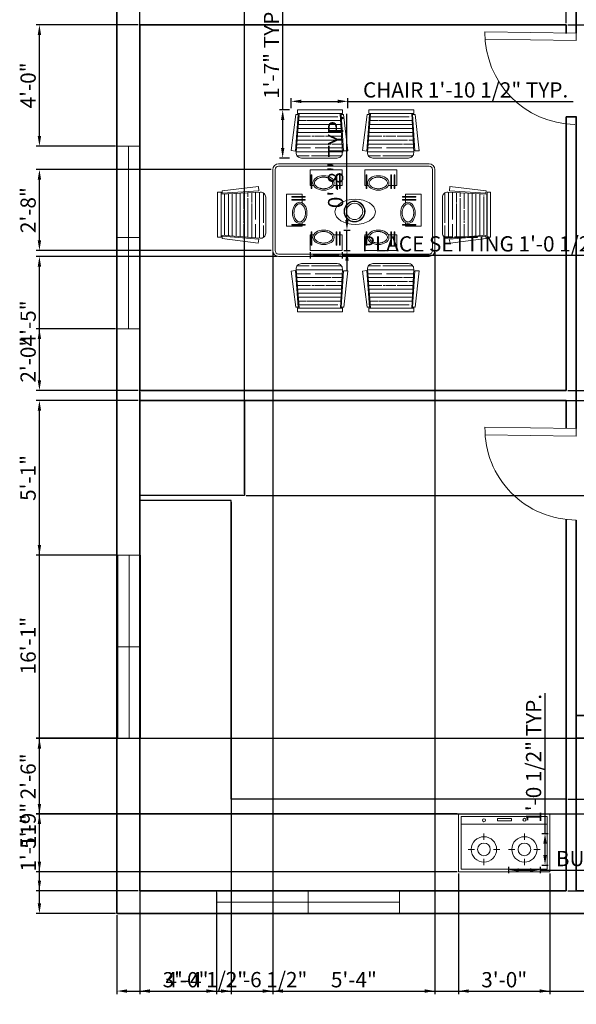
# Model space of a CAD drawing. Units: inches. Extents: x 1973 to 2661, y 1730 to 2412.
# Tile 1 of 5: x 1978 to 2197, y 1730 to 2117. Entities that reach past the tile are written whole.
import ezdxf

# ---------------------------------------------------------------- set-up
doc = ezdxf.new("R2010")
doc.units = ezdxf.units.IN
for name, color, linetype, lineweight in [('A-ANNO-DIMS', 2, 'Continuous', 18), ('A-DOOR', 3, 'Continuous', 18), ('A-EQPM', 9, 'Continuous', 18), ('A-FLOR-CASE', 32, 'Continuous', 25), ('A-FURN', 8, 'Continuous', 18), ('A-GLAZ', 4, 'Continuous', 18), ('A-WALL', 7, 'Continuous', 35)]:
    doc.layers.add(name, color=color, linetype=linetype, lineweight=lineweight)
doc.styles.get("Standard").update_dxf_attribs({"font": 'arial.ttf'})
doc.dimstyles.new('ISO-25', dxfattribs={"dimtxt": 6, "dimasz": 4, "dimexe": 1.25, "dimexo": 0.625, "dimtad": 1, "dimdec": 0, "dimrnd": 6, "dimlunit": 3, "dimtxsty": 'Standard', "dimcen": 2.5, "dimadec": 0, "dimazin": 0, "dimtfac": 1, "dimtdec": 0, "dimtmove": 0, "dimatfit": 3, "dimfxl": 1, "dimarcsym": 0})

# ---------------------------------------------------------------- blocks, each defined once
blk = doc.blocks.new('WIN-72-TWO-LIGHT')
for p, q in [((0, 72), (9, 72)), ((0, 0), (0, 72)), ((4.5, 72), (4.5, 36)), ((9, 72), (9, 0)), ((4.5, 36), (0, 36)), ((0, 36), (9, 36)), ((4.5, 36), (4.5, 0)), ((9, 0), (0, 0))]:
    blk.add_line(p, q)
blk = doc.blocks.new('CHAIR-DINING-SLATTED')
for p, q in [((0, 3.05), (1.85, 17.22)), ((2.79, 17.13), (1.68, 2.71)), ((1.85, 17.22), (2.79, 17.13)), ((1.98, 2.21), (3.17, 17.52)), ((2.47, 17.6), (2.47, 18.99)), ((2.47, 18.99), (20.19, 18.99)), ((20.19, 17.6), (2.47, 17.6)), ((3.07, 16.28), (18.38, 16.28)), ((18.88, 16.28), (18.96, 16.28)), ((19.37, 17.52), (20.16, 2.16)), ((20.68, 17.22), (19.74, 17.13)), ((19.74, 17.13), (20.61, 2.8)), ((20.19, 18.99), (20.19, 17.6)), ((22.33, 2.88), (20.68, 17.22)), ((2.72, 11.67), (19.67, 11.67)), ((2.83, 13.21), (19.59, 13.21)), ((2.95, 14.75), (6.04, 14.75)), ((6.28, 14.75), (19.51, 14.75)), ((2.48, 8.59), (7.56, 8.59)), ((2.6, 10.13), (19.75, 10.13)), ((8.13, 8.59), (8.91, 8.59)), ((9.16, 8.59), (13.09, 8.59)), ((13.59, 8.59), (19.83, 8.59)), ((2.12, 3.98), (7.56, 3.98)), ((2.24, 5.52), (15.72, 5.52)), ((2.36, 7.06), (17.73, 7.06)), ((9.4, 3.98), (20.07, 3.98)), ((16.09, 5.52), (19.99, 5.52)), ((18.26, 7.06), (19.91, 7.06)), ((1.68, 2.71), (0, 3.05)), ((2, 2.44), (20.15, 2.44)), ((2.33, 0.9), (7.06, 0.9)), ((18.11, 0), (4.03, 0)), ((8.05, 0.9), (19.81, 0.9)), ((20.61, 2.8), (22.33, 2.88))]:
    blk.add_line(p, q)
for centre, start, end in [((4.03, 2.05), 175.5808, 270), ((18.11, 2.05), 270, 2.9494)]:
    blk.add_arc(centre, 2.05, start, end)
blk = doc.blocks.new('DINING-PLACE-SETTING')
for p, q in [((0, 0), (0, 6.2)), ((0, 6.2), (1.33, 6.2)), ((0.44, 2.07), (0.44, 7.38)), ((0.44, 7.38), (0.7, 7.38)), ((0.7, 7.38), (0.7, 2.07)), ((9.19, 6.2), (12.59, 6.2)), ((10.26, 2.07), (10.26, 7.38)), ((10.26, 7.38), (10.52, 7.38)), ((10.52, 7.38), (10.52, 2.07)), ((11.48, 2.07), (11.48, 7.38)), ((11.48, 7.38), (11.74, 7.38)), ((11.74, 7.38), (11.74, 2.07)), ((12.59, 6.2), (12.59, 0)), ((12.59, 0), (0, 0)), ((0.7, 2.07), (0.44, 2.07)), ((10.52, 2.07), (10.26, 2.07)), ((11.74, 2.07), (11.48, 2.07))]:
    blk.add_line(p, q)
blk.add_ellipse((5.26, 5.21), major_axis=(4.19, 0), ratio=0.682819)
blk.add_open_spline([(8.86, 5.21), (8.86, 5.36), (8.83, 5.53), (8.71, 5.87), (8.6, 6.05), (8.39, 6.32), (8.3, 6.41), (8.11, 6.58), (8.01, 6.66), (7.66, 6.9), (7.39, 7.04), (6.95, 7.21), (6.8, 7.25), (6.5, 7.34), (6.34, 7.37), (6.03, 7.42), (5.87, 7.44), (5.56, 7.47), (5.42, 7.48), (5.1, 7.48), (4.96, 7.47), (4.65, 7.44), (4.49, 7.42), (4.18, 7.37), (4.03, 7.34), (3.72, 7.25), (3.57, 7.21), (3.13, 7.04), (2.86, 6.9), (2.52, 6.66), (2.41, 6.58), (2.22, 6.41), (2.14, 6.32), (1.92, 6.05), (1.82, 5.87), (1.69, 5.53), (1.66, 5.36), (1.66, 5.05), (1.69, 4.88), (1.82, 4.54), (1.92, 4.36), (2.14, 4.09), (2.22, 4), (2.41, 3.83), (2.52, 3.75), (2.86, 3.51), (3.13, 3.37), (3.57, 3.21), (3.72, 3.16), (4.03, 3.07), (4.18, 3.04), (4.49, 2.99), (4.65, 2.97), (4.96, 2.94), (5.1, 2.94), (5.42, 2.94), (5.56, 2.94), (5.87, 2.97), (6.03, 2.99), (6.34, 3.04), (6.5, 3.07), (6.8, 3.16), (6.95, 3.21), (7.39, 3.37), (7.66, 3.51), (8.01, 3.75), (8.11, 3.83), (8.3, 4), (8.39, 4.09), (8.6, 4.36), (8.71, 4.54), (8.83, 4.88), (8.86, 5.05), (8.86, 5.21)], degree=3, knots=[0, 0, 0, 0, 0.261799, 0.261799, 0.523599, 0.523599, 0.654498, 0.654498, 0.785398, 0.785398, 1.047198, 1.047198, 1.178097, 1.178097, 1.308997, 1.308997, 1.439897, 1.439897, 1.570796, 1.570796, 1.701696, 1.701696, 1.832596, 1.832596, 1.963495, 1.963495, 2.094395, 2.094395, 2.356194, 2.356194, 2.487094, 2.487094, 2.617994, 2.617994, 2.879793, 2.879793, 3.141593, 3.141593, 3.403392, 3.403392, 3.665191, 3.665191, 3.796091, 3.796091, 3.926991, 3.926991, 4.18879, 4.18879, 4.31969, 4.31969, 4.45059, 4.45059, 4.581489, 4.581489, 4.712389, 4.712389, 4.843289, 4.843289, 4.974188, 4.974188, 5.105088, 5.105088, 5.235988, 5.235988, 5.497787, 5.497787, 5.628687, 5.628687, 5.759587, 5.759587, 6.021386, 6.021386, 6.283185, 6.283185, 6.283185, 6.283185])
blk = doc.blocks.new('COOKTOP-BURNER')
for p, q in [((6.24, 9.98), (6.24, 12.48)), ((2.5, 6.24), (0, 6.24)), ((12.48, 6.24), (9.98, 6.24)), ((6.24, 0), (6.24, 2.5))]:
    blk.add_line(p, q)
for radius in [4.99, 2.5]:
    blk.add_circle((6.24, 6.24), radius)
blk = doc.blocks.new('*D16')
at = {"layer": 'A-ANNO-DIMS', "color": 0, "lineweight": -2, "transparency": 16777216}
for p, q in [((2092.18, 2025.82), (2092.18, 2023.31)), ((2096.18, 2024.56), (2100.77, 2024.56)), ((2104.77, 2025.82), (2104.77, 2023.31)), ((2104.77, 2024.56), (2228.74, 2024.56))]:
    blk.add_line(p, q, dxfattribs=at)
at = {"layer": 'A-ANNO-DIMS', "color": 0, "transparency": 16777216}
for points in [[(2096.18, 2025.23), (2096.18, 2023.89), (2092.18, 2024.56)], [(2100.77, 2025.23), (2100.77, 2023.89), (2104.77, 2024.56)]]:
    blk.add_solid(points, dxfattribs=at)
at = {"layer": 'Defpoints', "color": 0, "transparency": 16777216}
for p in [(2092.18, 2026.45), (2104.77, 2026.45), (2104.77, 2024.56)]:
    blk.add_point(p, dxfattribs=at)
at = {"layer": 'A-ANNO-DIMS', "color": 0, "transparency": 16777216, "insert": (2168.76, 2028.29), "char_height": 6, "attachment_point": 5}
blk.add_mtext('PLACE SETTING 1\'-0 1/2" TYP.', dxfattribs=at)
blk = doc.blocks.new('*D17')
at = {"layer": 'A-ANNO-DIMS', "color": 0, "lineweight": -2, "transparency": 16777216}
for p, q in [((2106.66, 2038.51), (2106.66, 2080.34)), ((2105.4, 2034.51), (2107.91, 2034.51)), ((2106.66, 2026.45), (2106.66, 2034.51)), ((2105.4, 2026.45), (2107.91, 2026.45)), ((2106.66, 2022.45), (2106.66, 2018.45))]:
    blk.add_line(p, q, dxfattribs=at)
at = {"layer": 'A-ANNO-DIMS', "color": 0, "transparency": 16777216}
for points in [[(2105.99, 2038.51), (2107.33, 2038.51), (2106.66, 2034.51)], [(2105.99, 2022.45), (2107.33, 2022.45), (2106.66, 2026.45)]]:
    blk.add_solid(points, dxfattribs=at)
at = {"layer": 'Defpoints', "color": 0, "transparency": 16777216}
for p in [(2104.77, 2034.51), (2106.66, 2034.51), (2104.77, 2026.45)]:
    blk.add_point(p, dxfattribs=at)
at = {"layer": 'A-ANNO-DIMS', "color": 0, "transparency": 16777216, "insert": (2102.97, 2061.43), "char_height": 6, "attachment_point": 5, "rotation": 90}
blk.add_mtext('0\'-8" TYP.', dxfattribs=at)
blk = doc.blocks.new('*D20')
at = {"layer": 'A-ANNO-DIMS', "color": 0, "lineweight": -2, "transparency": 16777216}
for p, q in [((2084.68, 2082.47), (2084.68, 2086.44)), ((2107.02, 2082.47), (2107.02, 2086.44)), ((2088.68, 2085.19), (2103.02, 2085.19)), ((2107.02, 2085.19), (2195.82, 2085.19))]:
    blk.add_line(p, q, dxfattribs=at)
at = {"layer": 'A-ANNO-DIMS', "color": 0, "transparency": 16777216}
for points in [[(2088.68, 2085.86), (2088.68, 2084.53), (2084.68, 2085.19)], [(2103.02, 2085.86), (2103.02, 2084.53), (2107.02, 2085.19)]]:
    blk.add_solid(points, dxfattribs=at)
at = {"layer": 'Defpoints', "color": 0, "transparency": 16777216}
for p in [(2107.02, 2085.19), (2084.68, 2081.84), (2107.02, 2081.84)]:
    blk.add_point(p, dxfattribs=at)
at = {"layer": 'A-ANNO-DIMS', "color": 0, "transparency": 16777216, "insert": (2153.42, 2088.92), "char_height": 6, "attachment_point": 5}
blk.add_mtext('CHAIR 1\'-10 1/2" TYP.', dxfattribs=at)
blk = doc.blocks.new('*D21')
at = {"layer": 'A-ANNO-DIMS', "color": 0, "lineweight": -2, "transparency": 16777216}
for p, q in [((2081.33, 2081.84), (2081.33, 2123.1)), ((2084.06, 2081.84), (2080.08, 2081.84)), ((2081.33, 2066.85), (2081.33, 2077.84)), ((2084.06, 2062.85), (2080.08, 2062.85))]:
    blk.add_line(p, q, dxfattribs=at)
at = {"layer": 'A-ANNO-DIMS', "color": 0, "transparency": 16777216}
for points in [[(2080.67, 2077.84), (2082, 2077.84), (2081.33, 2081.84)], [(2080.67, 2066.85), (2082, 2066.85), (2081.33, 2062.85)]]:
    blk.add_solid(points, dxfattribs=at)
at = {"layer": 'Defpoints', "color": 0, "transparency": 16777216}
for p in [(2081.33, 2081.84), (2084.68, 2081.84), (2084.68, 2062.85)]:
    blk.add_point(p, dxfattribs=at)
at = {"layer": 'A-ANNO-DIMS', "color": 0, "transparency": 16777216, "insert": (2077.7, 2104.47), "char_height": 6, "attachment_point": 5, "rotation": 90}
blk.add_mtext('1\'-7" TYP.', dxfattribs=at)
blk = doc.blocks.new('*D28')
at = {"layer": 'A-ANNO-DIMS', "color": 0, "lineweight": -2, "transparency": 16777216}
for p, q in [((2170.36, 1783.74), (2170.36, 1781.24)), ((2182.84, 1783.74), (2182.84, 1781.24)), ((2174.36, 1782.49), (2178.84, 1782.49)), ((2182.84, 1782.49), (2276.1, 1782.49))]:
    blk.add_line(p, q, dxfattribs=at)
at = {"layer": 'A-ANNO-DIMS', "color": 0, "transparency": 16777216}
for points in [[(2174.36, 1783.16), (2174.36, 1781.83), (2170.36, 1782.49)], [(2178.84, 1783.16), (2178.84, 1781.83), (2182.84, 1782.49)]]:
    blk.add_solid(points, dxfattribs=at)
at = {"layer": 'Defpoints', "color": 0, "transparency": 16777216}
for p in [(2170.36, 1784.36), (2182.84, 1784.36), (2182.84, 1782.49)]:
    blk.add_point(p, dxfattribs=at)
at = {"layer": 'A-ANNO-DIMS', "color": 0, "transparency": 16777216, "insert": (2231.47, 1786.22), "char_height": 6, "attachment_point": 5}
blk.add_mtext('BURNER 1\'-0 1/2" TYP.', dxfattribs=at)
blk = doc.blocks.new('*D29')
at = {"layer": 'A-ANNO-DIMS', "color": 0, "lineweight": -2, "transparency": 16777216}
for p, q in [((2184.71, 1796.84), (2184.71, 1852.08)), ((2183.47, 1796.84), (2185.96, 1796.84)), ((2184.71, 1788.36), (2184.71, 1792.84)), ((2183.47, 1784.36), (2185.96, 1784.36))]:
    blk.add_line(p, q, dxfattribs=at)
at = {"layer": 'A-ANNO-DIMS', "color": 0, "transparency": 16777216}
for points in [[(2184.05, 1792.84), (2185.38, 1792.84), (2184.71, 1796.84)], [(2184.05, 1788.36), (2185.38, 1788.36), (2184.71, 1784.36)]]:
    blk.add_solid(points, dxfattribs=at)
at = {"layer": 'Defpoints', "color": 0, "transparency": 16777216}
for p in [(2182.84, 1796.84), (2184.71, 1796.84), (2182.84, 1784.36)]:
    blk.add_point(p, dxfattribs=at)
at = {"layer": 'A-ANNO-DIMS', "color": 0, "transparency": 16777216, "insert": (2180.98, 1826.46), "char_height": 6, "attachment_point": 5, "rotation": 90}
blk.add_mtext('1\'-0 1/2" TYP.', dxfattribs=at)
blk = doc.blocks.new('*D30')
at = {"layer": 'A-ANNO-DIMS', "color": 0, "lineweight": -2, "transparency": 16777216}
for p, q in [((2016.04, 1764.73), (2016.04, 1733.57)), ((2616.04, 1764.73), (2616.04, 1733.57)), ((2020.04, 1734.82), (2612.04, 1734.82))]:
    blk.add_line(p, q, dxfattribs=at)
at = {"layer": 'A-ANNO-DIMS', "color": 0, "transparency": 16777216}
for points in [[(2020.04, 1735.49), (2020.04, 1734.15), (2016.04, 1734.82)], [(2612.04, 1735.49), (2612.04, 1734.15), (2616.04, 1734.82)]]:
    blk.add_solid(points, dxfattribs=at)
at = {"layer": 'Defpoints', "color": 0, "transparency": 16777216}
for p in [(2016.04, 1765.35), (2616.04, 1765.35), (2616.04, 1734.82)]:
    blk.add_point(p, dxfattribs=at)
at = {"layer": 'A-ANNO-DIMS', "color": 0, "transparency": 16777216, "insert": (2316.04, 1738.51), "char_height": 6, "attachment_point": 5}
blk.add_mtext('50\'-0"', dxfattribs=at)
blk = doc.blocks.new('*D40')
at = {"layer": 'A-ANNO-DIMS', "color": 0, "lineweight": -2, "transparency": 16777216}
for p, q in [((2015.71, 1834.42), (1984.22, 1834.42)), ((1985.47, 1769.35), (1985.47, 1830.42)), ((2015.42, 1765.35), (1984.22, 1765.35))]:
    blk.add_line(p, q, dxfattribs=at)
at = {"layer": 'A-ANNO-DIMS', "color": 0, "transparency": 16777216}
for points in [[(1984.81, 1830.42), (1986.14, 1830.42), (1985.47, 1834.42)], [(1984.81, 1769.35), (1986.14, 1769.35), (1985.47, 1765.35)]]:
    blk.add_solid(points, dxfattribs=at)
at = {"layer": 'Defpoints', "color": 0, "transparency": 16777216}
for p in [(1985.47, 1834.42), (2016.33, 1834.42), (2016.04, 1765.35)]:
    blk.add_point(p, dxfattribs=at)
at = {"layer": 'A-ANNO-DIMS', "color": 0, "transparency": 16777216, "insert": (1981.79, 1799.89), "char_height": 6, "attachment_point": 5, "rotation": 90}
blk.add_mtext('5\'-9"', dxfattribs=at)
blk = doc.blocks.new('*D41')
at = {"layer": 'A-ANNO-DIMS', "color": 0, "lineweight": -2, "transparency": 16777216}
for p, q in [((2024.42, 1967.35), (1984.22, 1967.35)), ((1985.47, 1910.42), (1985.47, 1963.35)), ((2015.71, 1906.42), (1984.22, 1906.42))]:
    blk.add_line(p, q, dxfattribs=at)
at = {"layer": 'A-ANNO-DIMS', "color": 0, "transparency": 16777216}
for points in [[(1984.81, 1963.35), (1986.14, 1963.35), (1985.47, 1967.35)], [(1984.81, 1910.42), (1986.14, 1910.42), (1985.47, 1906.42)]]:
    blk.add_solid(points, dxfattribs=at)
at = {"layer": 'Defpoints', "color": 0, "transparency": 16777216}
for p in [(1985.47, 1967.35), (2025.04, 1967.35), (2016.33, 1906.42)]:
    blk.add_point(p, dxfattribs=at)
at = {"layer": 'A-ANNO-DIMS', "color": 0, "transparency": 16777216, "insert": (1981.79, 1936.89), "char_height": 6, "attachment_point": 5, "rotation": 90}
blk.add_mtext('5\'-1"', dxfattribs=at)
blk = doc.blocks.new('*D42')
at = {"layer": 'A-ANNO-DIMS', "color": 0, "lineweight": -2, "transparency": 16777216}
for p, q in [((2015.49, 1995.59), (1984.22, 1995.59)), ((1985.47, 1975.35), (1985.47, 1991.59)), ((2024.42, 1971.35), (1984.22, 1971.35))]:
    blk.add_line(p, q, dxfattribs=at)
at = {"layer": 'A-ANNO-DIMS', "color": 0, "transparency": 16777216}
for points in [[(1984.81, 1991.59), (1986.14, 1991.59), (1985.47, 1995.59)], [(1984.81, 1975.35), (1986.14, 1975.35), (1985.47, 1971.35)]]:
    blk.add_solid(points, dxfattribs=at)
at = {"layer": 'Defpoints', "color": 0, "transparency": 16777216}
for p in [(1985.47, 1995.59), (2016.11, 1995.59), (2025.04, 1971.35)]:
    blk.add_point(p, dxfattribs=at)
at = {"layer": 'A-ANNO-DIMS', "color": 0, "transparency": 16777216, "insert": (1981.79, 1983.47), "char_height": 6, "attachment_point": 5, "rotation": 90}
blk.add_mtext('2\'-0"', dxfattribs=at)
blk = doc.blocks.new('*D43')
at = {"layer": 'A-ANNO-DIMS', "color": 0, "lineweight": -2, "transparency": 16777216}
for p, q in [((2024.42, 2115.35), (1984.22, 2115.35)), ((1985.47, 2071.59), (1985.47, 2111.35)), ((2015.49, 2067.59), (1984.22, 2067.59))]:
    blk.add_line(p, q, dxfattribs=at)
at = {"layer": 'A-ANNO-DIMS', "color": 0, "transparency": 16777216}
for points in [[(1984.81, 2111.35), (1986.14, 2111.35), (1985.47, 2115.35)], [(1984.81, 2071.59), (1986.14, 2071.59), (1985.47, 2067.59)]]:
    blk.add_solid(points, dxfattribs=at)
at = {"layer": 'Defpoints', "color": 0, "transparency": 16777216}
for p in [(1985.47, 2115.35), (2025.04, 2115.35), (2016.11, 2067.59)]:
    blk.add_point(p, dxfattribs=at)
at = {"layer": 'A-ANNO-DIMS', "color": 0, "transparency": 16777216, "insert": (1981.79, 2091.47), "char_height": 6, "attachment_point": 5, "rotation": 90}
blk.add_mtext('4\'-0"', dxfattribs=at)
blk = doc.blocks.new('*D46')
at = {"layer": 'A-ANNO-DIMS', "color": 0, "lineweight": -2, "transparency": 16777216}
for p, q in [((2025.04, 2115.98), (2025.04, 2397.1)), ((2193.04, 2115.98), (2193.04, 2397.1)), ((2029.04, 2395.85), (2189.04, 2395.85))]:
    blk.add_line(p, q, dxfattribs=at)
at = {"layer": 'A-ANNO-DIMS', "color": 0, "transparency": 16777216}
for points in [[(2029.04, 2396.52), (2029.04, 2395.18), (2025.04, 2395.85)], [(2189.04, 2396.52), (2189.04, 2395.18), (2193.04, 2395.85)]]:
    blk.add_solid(points, dxfattribs=at)
at = {"layer": 'Defpoints', "color": 0, "transparency": 16777216}
for p in [(2193.04, 2395.85), (2025.04, 2115.35), (2193.04, 2115.35)]:
    blk.add_point(p, dxfattribs=at)
at = {"layer": 'A-ANNO-DIMS', "color": 0, "transparency": 16777216, "insert": (2109.04, 2399.54), "char_height": 6, "attachment_point": 5}
blk.add_mtext('14\'-0"', dxfattribs=at)
blk = doc.blocks.new('*D55')
at = {"layer": 'A-ANNO-DIMS', "color": 0, "lineweight": -2, "transparency": 16777216}
for p, q in [((2025.04, 1927.35), (2025.04, 1733.57)), ((2061.04, 1927.35), (2061.04, 1733.57)), ((2029.04, 1734.82), (2057.04, 1734.82))]:
    blk.add_line(p, q, dxfattribs=at)
at = {"layer": 'A-ANNO-DIMS', "color": 0, "transparency": 16777216}
for points in [[(2029.04, 1735.49), (2029.04, 1734.15), (2025.04, 1734.82)], [(2057.04, 1735.49), (2057.04, 1734.15), (2061.04, 1734.82)]]:
    blk.add_solid(points, dxfattribs=at)
at = {"layer": 'Defpoints', "color": 0, "transparency": 16777216}
for p in [(2025.04, 1927.97), (2061.04, 1927.97), (2061.04, 1734.82)]:
    blk.add_point(p, dxfattribs=at)
at = {"layer": 'A-ANNO-DIMS', "color": 0, "transparency": 16777216, "insert": (2043.04, 1738.51), "char_height": 6, "attachment_point": 5}
blk.add_mtext('3\'-0"', dxfattribs=at)
blk = doc.blocks.new('*D56')
at = {"layer": 'A-ANNO-DIMS', "color": 0, "lineweight": -2, "transparency": 16777216}
for p, q in [((2025.04, 1773.73), (2025.04, 1733.57)), ((2055.31, 1773.69), (2055.31, 1733.57)), ((2029.04, 1734.82), (2051.31, 1734.82)), ((2055.31, 1734.82), (2090.6, 1734.82))]:
    blk.add_line(p, q, dxfattribs=at)
at = {"layer": 'A-ANNO-DIMS', "color": 0, "transparency": 16777216}
for points in [[(2029.04, 1735.49), (2029.04, 1734.15), (2025.04, 1734.82)], [(2051.31, 1735.49), (2051.31, 1734.15), (2055.31, 1734.82)]]:
    blk.add_solid(points, dxfattribs=at)
at = {"layer": 'Defpoints', "color": 0, "transparency": 16777216}
for p in [(2025.04, 1774.35), (2055.31, 1774.32), (2055.31, 1734.82)]:
    blk.add_point(p, dxfattribs=at)
at = {"layer": 'A-ANNO-DIMS', "color": 0, "transparency": 16777216, "insert": (2074.95, 1738.55), "char_height": 6, "attachment_point": 5}
blk.add_mtext('2\'-6 1/2"', dxfattribs=at)
blk = doc.blocks.new('*D57')
at = {"layer": 'A-ANNO-DIMS', "color": 0, "lineweight": -2, "transparency": 16777216}
for p, q in [((2193.67, 1810.35), (2647.79, 1810.35)), ((2646.54, 1778.35), (2646.54, 1806.35)), ((2193.67, 1774.35), (2647.79, 1774.35))]:
    blk.add_line(p, q, dxfattribs=at)
at = {"layer": 'A-ANNO-DIMS', "color": 0, "transparency": 16777216}
for points in [[(2645.88, 1806.35), (2647.21, 1806.35), (2646.54, 1810.35)], [(2645.88, 1778.35), (2647.21, 1778.35), (2646.54, 1774.35)]]:
    blk.add_solid(points, dxfattribs=at)
at = {"layer": 'Defpoints', "color": 0, "transparency": 16777216}
for p in [(2193.04, 1810.35), (2646.54, 1810.35), (2193.04, 1774.35)]:
    blk.add_point(p, dxfattribs=at)
at = {"layer": 'A-ANNO-DIMS', "color": 0, "transparency": 16777216, "insert": (2642.85, 1792.35), "char_height": 6, "attachment_point": 5, "rotation": 90}
blk.add_mtext('3\'-0"', dxfattribs=at)
blk = doc.blocks.new('*D58')
at = {"layer": 'A-ANNO-DIMS', "color": 0, "lineweight": -2, "transparency": 16777216}
for p, q in [((2024.42, 1967.35), (1984.22, 1967.35)), ((1985.47, 1778.35), (1985.47, 1963.35)), ((2024.42, 1774.35), (1984.22, 1774.35))]:
    blk.add_line(p, q, dxfattribs=at)
at = {"layer": 'A-ANNO-DIMS', "color": 0, "transparency": 16777216}
for points in [[(1984.81, 1963.35), (1986.14, 1963.35), (1985.47, 1967.35)], [(1984.81, 1778.35), (1986.14, 1778.35), (1985.47, 1774.35)]]:
    blk.add_solid(points, dxfattribs=at)
at = {"layer": 'Defpoints', "color": 0, "transparency": 16777216}
for p in [(1985.47, 1967.35), (2025.04, 1967.35), (2025.04, 1774.35)]:
    blk.add_point(p, dxfattribs=at)
at = {"layer": 'A-ANNO-DIMS', "color": 0, "transparency": 16777216, "insert": (1981.79, 1870.85), "char_height": 6, "attachment_point": 5, "rotation": 90}
blk.add_mtext('16\'-1"', dxfattribs=at)
blk = doc.blocks.new('*D59')
at = {"layer": 'A-ANNO-DIMS', "color": 0, "lineweight": -2, "transparency": 16777216}
for p, q in [((2193.67, 2115.35), (2647.79, 2115.35)), ((2646.54, 1975.35), (2646.54, 2111.35)), ((2193.67, 1971.35), (2647.79, 1971.35))]:
    blk.add_line(p, q, dxfattribs=at)
at = {"layer": 'A-ANNO-DIMS', "color": 0, "transparency": 16777216}
for points in [[(2645.88, 2111.35), (2647.21, 2111.35), (2646.54, 2115.35)], [(2645.88, 1975.35), (2647.21, 1975.35), (2646.54, 1971.35)]]:
    blk.add_solid(points, dxfattribs=at)
at = {"layer": 'Defpoints', "color": 0, "transparency": 16777216}
for p in [(2193.04, 2115.35), (2646.54, 2115.35), (2193.04, 1971.35)]:
    blk.add_point(p, dxfattribs=at)
at = {"layer": 'A-ANNO-DIMS', "color": 0, "transparency": 16777216, "insert": (2642.85, 2043.35), "char_height": 6, "attachment_point": 5, "rotation": 90}
blk.add_mtext('12\'-0"', dxfattribs=at)
blk = doc.blocks.new('*D64')
at = {"layer": 'A-ANNO-DIMS', "color": 0, "lineweight": -2, "transparency": 16777216}
for p, q in [((2324.17, 1834.25), (1984.22, 1834.25)), ((1985.47, 1808.45), (1985.47, 1830.25)), ((2324.17, 1804.45), (1984.22, 1804.45))]:
    blk.add_line(p, q, dxfattribs=at)
at = {"layer": 'A-ANNO-DIMS', "color": 0, "transparency": 16777216}
for points in [[(1984.81, 1830.25), (1986.14, 1830.25), (1985.47, 1834.25)], [(1984.81, 1808.45), (1986.14, 1808.45), (1985.47, 1804.45)]]:
    blk.add_solid(points, dxfattribs=at)
at = {"layer": 'Defpoints', "color": 0, "transparency": 16777216}
for p in [(1985.47, 1834.25), (2324.79, 1834.25), (2324.79, 1804.45)]:
    blk.add_point(p, dxfattribs=at)
at = {"layer": 'A-ANNO-DIMS', "color": 0, "transparency": 16777216, "insert": (1981.79, 1819.35), "char_height": 6, "attachment_point": 5, "rotation": 90}
blk.add_mtext('2\'-6"', dxfattribs=at)
blk = doc.blocks.new('*D70')
at = {"layer": 'A-ANNO-DIMS', "color": 0, "lineweight": -2, "transparency": 16777216}
for p, q in [((2077.47, 2025.78), (2077.47, 1733.57)), ((2141.28, 2025.78), (2141.28, 1733.57)), ((2081.47, 1734.82), (2137.28, 1734.82))]:
    blk.add_line(p, q, dxfattribs=at)
at = {"layer": 'A-ANNO-DIMS', "color": 0, "transparency": 16777216}
for points in [[(2081.47, 1735.49), (2081.47, 1734.15), (2077.47, 1734.82)], [(2137.28, 1735.49), (2137.28, 1734.15), (2141.28, 1734.82)]]:
    blk.add_solid(points, dxfattribs=at)
at = {"layer": 'Defpoints', "color": 0, "transparency": 16777216}
for p in [(2077.47, 2026.4), (2141.28, 2026.4), (2141.28, 1734.82)]:
    blk.add_point(p, dxfattribs=at)
at = {"layer": 'A-ANNO-DIMS', "color": 0, "transparency": 16777216, "insert": (2109.38, 1738.5), "char_height": 6, "attachment_point": 5}
blk.add_mtext('5\'-4"', dxfattribs=at)
blk = doc.blocks.new('*D71')
at = {"layer": 'A-ANNO-DIMS', "color": 0, "lineweight": -2, "transparency": 16777216}
for p, q in [((2076.85, 2058.31), (1984.22, 2058.31)), ((1985.47, 2030.4), (1985.47, 2054.31)), ((2076.85, 2026.4), (1984.22, 2026.4))]:
    blk.add_line(p, q, dxfattribs=at)
at = {"layer": 'A-ANNO-DIMS', "color": 0, "transparency": 16777216}
for points in [[(1984.81, 2054.31), (1986.14, 2054.31), (1985.47, 2058.31)], [(1984.81, 2030.4), (1986.14, 2030.4), (1985.47, 2026.4)]]:
    blk.add_solid(points, dxfattribs=at)
at = {"layer": 'Defpoints', "color": 0, "transparency": 16777216}
for p in [(1985.47, 2058.31), (2077.47, 2058.31), (2077.47, 2026.4)]:
    blk.add_point(p, dxfattribs=at)
at = {"layer": 'A-ANNO-DIMS', "color": 0, "transparency": 16777216, "insert": (1981.79, 2042.35), "char_height": 6, "attachment_point": 5, "rotation": 90}
blk.add_mtext('2\'-8"', dxfattribs=at)
blk = doc.blocks.new('*D72')
at = {"layer": 'A-ANNO-DIMS', "color": 0, "lineweight": -2, "transparency": 16777216}
for p, q in [((2025.04, 1930.6), (2025.04, 2397.1)), ((2066.26, 1930.6), (2066.26, 2397.1)), ((2062.26, 2395.85), (2029.04, 2395.85))]:
    blk.add_line(p, q, dxfattribs=at)
at = {"layer": 'A-ANNO-DIMS', "color": 0, "transparency": 16777216}
for points in [[(2029.04, 2396.52), (2029.04, 2395.18), (2025.04, 2395.85)], [(2062.26, 2396.52), (2062.26, 2395.18), (2066.26, 2395.85)]]:
    blk.add_solid(points, dxfattribs=at)
at = {"layer": 'Defpoints', "color": 0, "transparency": 16777216}
for p in [(2025.04, 2395.85), (2025.04, 1929.97), (2066.26, 1929.97)]:
    blk.add_point(p, dxfattribs=at)
at = {"layer": 'A-ANNO-DIMS', "color": 0, "transparency": 16777216, "insert": (2045.65, 2399.54), "char_height": 6, "attachment_point": 5}
blk.add_mtext('3\'-5"', dxfattribs=at)
blk = doc.blocks.new('*D73')
at = {"layer": 'A-ANNO-DIMS', "color": 0, "lineweight": -2, "transparency": 16777216}
for p, q in [((2066.89, 1967.35), (2647.79, 1967.35)), ((2646.54, 1933.97), (2646.54, 1963.35)), ((2066.89, 1929.97), (2647.79, 1929.97))]:
    blk.add_line(p, q, dxfattribs=at)
at = {"layer": 'A-ANNO-DIMS', "color": 0, "transparency": 16777216}
for points in [[(2645.88, 1963.35), (2647.21, 1963.35), (2646.54, 1967.35)], [(2645.88, 1933.97), (2647.21, 1933.97), (2646.54, 1929.97)]]:
    blk.add_solid(points, dxfattribs=at)
at = {"layer": 'Defpoints', "color": 0, "transparency": 16777216}
for p in [(2066.26, 1967.35), (2646.54, 1967.35), (2066.26, 1929.97)]:
    blk.add_point(p, dxfattribs=at)
at = {"layer": 'A-ANNO-DIMS', "color": 0, "transparency": 16777216, "insert": (2642.81, 1948.66), "char_height": 6, "attachment_point": 5, "rotation": 90}
blk.add_mtext('3\'-1 1/2"', dxfattribs=at)
blk = doc.blocks.new('*D74')
at = {"layer": 'A-ANNO-DIMS', "color": 0, "lineweight": -2, "transparency": 16777216}
for p, q in [((2150.66, 1781.14), (2150.66, 1733.57)), ((2186.58, 1781.14), (2186.58, 1733.57)), ((2154.66, 1734.82), (2182.58, 1734.82))]:
    blk.add_line(p, q, dxfattribs=at)
at = {"layer": 'A-ANNO-DIMS', "color": 0, "transparency": 16777216}
for points in [[(2154.66, 1735.49), (2154.66, 1734.15), (2150.66, 1734.82)], [(2182.58, 1735.49), (2182.58, 1734.15), (2186.58, 1734.82)]]:
    blk.add_solid(points, dxfattribs=at)
at = {"layer": 'Defpoints', "color": 0, "transparency": 16777216}
for p in [(2150.66, 1781.77), (2186.58, 1781.77), (2186.58, 1734.82)]:
    blk.add_point(p, dxfattribs=at)
at = {"layer": 'A-ANNO-DIMS', "color": 0, "transparency": 16777216, "insert": (2168.62, 1738.51), "char_height": 6, "attachment_point": 5}
blk.add_mtext('3\'-0"', dxfattribs=at)
blk = doc.blocks.new('*D75')
at = {"layer": 'A-ANNO-DIMS', "color": 0, "lineweight": -2, "transparency": 16777216}
for p, q in [((2150.04, 1804.58), (1984.22, 1804.58)), ((1985.47, 1785.77), (1985.47, 1800.58)), ((2150.04, 1781.77), (1984.22, 1781.77))]:
    blk.add_line(p, q, dxfattribs=at)
at = {"layer": 'A-ANNO-DIMS', "color": 0, "transparency": 16777216}
for points in [[(1984.81, 1800.58), (1986.14, 1800.58), (1985.47, 1804.58)], [(1984.81, 1785.77), (1986.14, 1785.77), (1985.47, 1781.77)]]:
    blk.add_solid(points, dxfattribs=at)
at = {"layer": 'Defpoints', "color": 0, "transparency": 16777216}
for p in [(1985.47, 1804.58), (2150.66, 1804.58), (2150.66, 1781.77)]:
    blk.add_point(p, dxfattribs=at)
at = {"layer": 'A-ANNO-DIMS', "color": 0, "transparency": 16777216, "insert": (1981.84, 1793.17), "char_height": 6, "attachment_point": 5, "rotation": 90}
blk.add_mtext('1\'-11"', dxfattribs=at)
blk = doc.blocks.new('*D78')
at = {"layer": 'A-ANNO-DIMS', "color": 0, "lineweight": -2, "transparency": 16777216}
for p, q in [((2077.47, 2025.78), (2077.47, 1733.57)), ((2025.04, 1970.73), (2025.04, 1733.57)), ((2029.04, 1734.82), (2073.47, 1734.82))]:
    blk.add_line(p, q, dxfattribs=at)
at = {"layer": 'A-ANNO-DIMS', "color": 0, "transparency": 16777216}
for points in [[(2029.04, 1735.49), (2029.04, 1734.15), (2025.04, 1734.82)], [(2073.47, 1735.49), (2073.47, 1734.15), (2077.47, 1734.82)]]:
    blk.add_solid(points, dxfattribs=at)
at = {"layer": 'Defpoints', "color": 0, "transparency": 16777216}
for p in [(2077.47, 2026.4), (2025.04, 1971.35), (2077.47, 1734.82)]:
    blk.add_point(p, dxfattribs=at)
at = {"layer": 'A-ANNO-DIMS', "color": 0, "transparency": 16777216, "insert": (2051.26, 1738.55), "char_height": 6, "attachment_point": 5}
blk.add_mtext('4\'-4 1/2"', dxfattribs=at)
blk = doc.blocks.new('*D79')
at = {"layer": 'A-ANNO-DIMS', "color": 0, "lineweight": -2, "transparency": 16777216}
for p, q in [((2079.13, 2024.12), (1984.22, 2024.12)), ((1985.47, 1975.35), (1985.47, 2020.12)), ((2024.42, 1971.35), (1984.22, 1971.35))]:
    blk.add_line(p, q, dxfattribs=at)
at = {"layer": 'A-ANNO-DIMS', "color": 0, "transparency": 16777216}
for points in [[(1984.81, 2020.12), (1986.14, 2020.12), (1985.47, 2024.12)], [(1984.81, 1975.35), (1986.14, 1975.35), (1985.47, 1971.35)]]:
    blk.add_solid(points, dxfattribs=at)
at = {"layer": 'Defpoints', "color": 0, "transparency": 16777216}
for p in [(1985.47, 2024.12), (2079.75, 2024.12), (2025.04, 1971.35)]:
    blk.add_point(p, dxfattribs=at)
at = {"layer": 'A-ANNO-DIMS', "color": 0, "transparency": 16777216, "insert": (1981.8, 1997.74), "char_height": 6, "attachment_point": 5, "rotation": 90}
blk.add_mtext('4\'-5"', dxfattribs=at)

msp = doc.modelspace()

# ---------------------------------------------------------------- linework, layer by layer
at = {"layer": 'A-DOOR'}
for p, q in [((2161, 2109.63), (2197, 2109.1)), ((2197.04, 2112.1), (2161.05, 2112.62)), ((2161.05, 2112.62), (2197.04, 2112.1)), ((2197.04, 2109.1), (2197.04, 2112.1)), ((2197.04, 1956.32), (2161.05, 1956.84)), ((2161.05, 1956.84), (2197.04, 1956.32)), ((2197.04, 1956.32), (2197.04, 1953.31)), ((2161, 1953.84), (2197, 1953.32))]:
    msp.add_line(p, q, dxfattribs=at)
for centre, end in [((2197.04, 2112.1), 269.1676), ((2197.04, 1956.32), 270)]:
    msp.add_arc(centre, 36, 179.1676, end, dxfattribs=at)
at = {"layer": 'A-EQPM'}
for p, q in [((2150.66, 1781.77), (2150.66, 1804.58)), ((2150.66, 1804.58), (2186.58, 1804.58)), ((2151.66, 1782.76), (2151.66, 1803.58)), ((2151.66, 1803.58), (2185.59, 1803.58)), ((2185.59, 1803.58), (2185.59, 1782.76)), ((2186.58, 1804.58), (2186.58, 1781.77)), ((2185.59, 1800.59), (2151.66, 1800.59)), ((2166.02, 1802.71), (2171.53, 1802.71)), ((2166.02, 1801.91), (2166.02, 1802.71)), ((2171.53, 1801.91), (2166.02, 1801.91)), ((2171.53, 1802.71), (2171.53, 1801.91)), ((2186.58, 1781.77), (2150.66, 1781.77)), ((2185.59, 1782.76), (2151.66, 1782.76))]:
    msp.add_line(p, q, dxfattribs=at)
for centre in [(2160.65, 1802.09), (2176.63, 1802.27)]:
    msp.add_circle(centre, 0.599, dxfattribs=at)
at = {"layer": 'A-FLOR-CASE'}
for p, q in [((2025.04, 1929.97), (2025.04, 1967.35)), ((2025.04, 1967.35), (2066.26, 1967.35)), ((2066.26, 1967.35), (2066.26, 1929.97)), ((2066.26, 1929.97), (2025.04, 1929.97)), ((2061.04, 1927.97), (2025.04, 1927.97)), ((2061.04, 1810.35), (2061.04, 1927.97)), ((2193.04, 1810.35), (2061.04, 1810.35))]:
    msp.add_line(p, q, dxfattribs=at)
at = {"layer": 'A-FURN'}
for p, q in [((2079.75, 2060.58), (2139, 2060.58)), ((2079.75, 2059.67), (2139, 2059.67)), ((2077.47, 2026.4), (2077.47, 2058.31)), ((2078.38, 2058.31), (2078.38, 2026.4)), ((2140.37, 2058.31), (2140.37, 2026.4)), ((2141.28, 2058.31), (2141.28, 2026.4)), ((2071.78, 2051.61), (2057.44, 2049.97)), ((2071.87, 2049.9), (2071.78, 2051.61)), ((2147.07, 2049.9), (2147.15, 2051.61)), ((2147.15, 2051.61), (2161.49, 2049.97)), ((2055.67, 2031.75), (2055.67, 2049.47)), ((2055.67, 2049.47), (2057.07, 2049.47)), ((2057.07, 2049.47), (2057.07, 2031.75)), ((2057.15, 2048.65), (2072.51, 2049.44)), ((2057.44, 2049.97), (2057.53, 2049.03)), ((2057.53, 2049.03), (2071.87, 2049.9)), ((2058.38, 2032.36), (2058.38, 2048.72)), ((2059.92, 2035.57), (2059.92, 2048.8)), ((2061.45, 2032.12), (2061.45, 2048.87)), ((2062.99, 2032), (2062.99, 2048.95)), ((2064.53, 2031.88), (2064.53, 2049.03)), ((2066.07, 2042.87), (2066.07, 2049.11)), ((2067.61, 2047.55), (2067.61, 2049.19)), ((2069.15, 2045.37), (2069.15, 2049.27)), ((2070.68, 2038.69), (2070.68, 2049.35)), ((2072.22, 2031.29), (2072.22, 2049.43)), ((2073.76, 2037.33), (2073.76, 2049.09)), ((2074.66, 2033.31), (2074.66, 2047.4)), ((2144.27, 2047.4), (2144.27, 2033.31)), ((2145.17, 2037.33), (2145.17, 2049.09)), ((2161.78, 2048.65), (2146.43, 2049.44)), ((2146.71, 2031.29), (2146.71, 2049.43)), ((2161.4, 2049.03), (2147.07, 2049.9)), ((2148.25, 2038.69), (2148.25, 2049.35)), ((2149.79, 2045.37), (2149.79, 2049.27)), ((2151.32, 2047.55), (2151.32, 2049.19)), ((2152.86, 2042.87), (2152.86, 2049.11)), ((2154.4, 2031.88), (2154.4, 2049.03)), ((2155.94, 2032), (2155.94, 2048.95)), ((2157.48, 2032.12), (2157.48, 2048.87)), ((2159.01, 2035.57), (2159.01, 2048.8)), ((2160.55, 2048.16), (2160.55, 2048.24)), ((2160.55, 2032.36), (2160.55, 2047.67)), ((2161.49, 2049.97), (2161.4, 2049.03)), ((2161.78, 2032.45), (2161.78, 2048.65)), ((2161.87, 2049.47), (2161.87, 2031.75)), ((2163.26, 2049.47), (2161.87, 2049.47)), ((2163.26, 2031.75), (2163.26, 2049.47)), ((2067.61, 2031.64), (2067.61, 2047.01)), ((2069.15, 2031.52), (2069.15, 2045)), ((2149.79, 2031.52), (2149.79, 2045)), ((2151.32, 2031.64), (2151.32, 2047.01)), ((2066.07, 2038.44), (2066.07, 2042.38)), ((2152.86, 2038.44), (2152.86, 2042.38)), ((2066.07, 2037.41), (2066.07, 2038.19)), ((2066.07, 2031.76), (2066.07, 2036.84)), ((2070.68, 2031.4), (2070.68, 2036.84)), ((2073.76, 2031.61), (2073.76, 2036.35)), ((2145.17, 2031.61), (2145.17, 2036.35)), ((2148.25, 2031.4), (2148.25, 2036.84)), ((2152.86, 2037.41), (2152.86, 2038.19)), ((2152.86, 2031.76), (2152.86, 2036.84)), ((2072.45, 2031.27), (2057.15, 2032.45)), ((2057.44, 2031.14), (2057.53, 2032.08)), ((2057.53, 2032.08), (2071.95, 2030.96)), ((2059.92, 2032.24), (2059.92, 2035.32)), ((2146.48, 2031.27), (2161.78, 2032.45)), ((2161.4, 2032.08), (2146.98, 2030.96)), ((2159.01, 2032.24), (2159.01, 2035.32)), ((2161.49, 2031.14), (2161.4, 2032.08)), ((2057.07, 2031.75), (2055.67, 2031.75)), ((2071.62, 2029.28), (2057.44, 2031.14)), ((2071.95, 2030.96), (2071.62, 2029.28)), ((2146.98, 2030.96), (2147.32, 2029.28)), ((2147.32, 2029.28), (2161.49, 2031.14)), ((2161.87, 2031.75), (2163.26, 2031.75)), ((2139, 2025.04), (2079.75, 2025.04)), ((2139, 2024.12), (2079.75, 2024.12))]:
    msp.add_line(p, q, dxfattribs=at)
for radius in [4.13, 3.95, 3.21]:
    msp.add_circle((2109.65, 2041.84), radius, dxfattribs=at)
for centre, radius, start, end in [((2079.75, 2058.31), 2.28, 90, 180), ((2079.75, 2058.31), 1.37, 90, 180), ((2139, 2058.31), 2.28, 0, 90), ((2139, 2058.31), 1.37, 360, 90), ((2072.61, 2047.4), 2.05, 360, 92.9494), ((2146.32, 2047.4), 2.05, 87.0506, 180), ((2072.61, 2033.31), 2.05, 265.5808, 0), ((2146.32, 2033.31), 2.05, 180, 274.4192), ((2079.75, 2026.4), 2.28, 180, 270), ((2079.75, 2026.4), 1.37, 180, 270), ((2139, 2026.4), 2.28, 270, 0), ((2139, 2026.4), 1.37, 270, 0)]:
    msp.add_arc(centre, radius, start, end, dxfattribs=at)
msp.add_ellipse((2109.89, 2041.69), major_axis=(-7.96, 0), ratio=0.62413, dxfattribs=at)
at = {"layer": 'A-WALL'}
for p, q in [((2016.04, 1765.35), (2016.04, 2365.35)), ((2197.04, 2112.1), (2197.04, 2125.17)), ((2193.04, 2115.35), (2025.04, 2115.35)), ((2025.04, 2115.35), (2025.04, 1971.35)), ((2193.04, 2111.88), (2193.04, 2115.35)), ((2193.04, 2115.35), (2193.04, 2112.1)), ((2193.04, 1971.35), (2193.04, 2079.16)), ((2193.04, 2079.16), (2197.09, 2079.1)), ((2197.04, 2076.1), (2197.04, 2079.1)), ((2197.04, 2079.1), (2197.04, 1956.32)), ((2025.04, 1971.35), (2193.04, 1971.35)), ((2193.04, 1967.35), (2025.04, 1967.35)), ((2025.04, 1967.35), (2025.04, 1774.35)), ((2193.04, 1956.37), (2193.04, 1967.35)), ((2193.04, 1967.35), (2193.04, 1956.32)), ((2193.04, 1774.35), (2193.04, 1920.54)), ((2197.04, 1920.32), (2197.04, 1834.35)), ((2370.04, 1843.35), (2197.04, 1843.35)), ((2197.04, 1834.35), (2499.04, 1834.35)), ((2197.04, 1834.35), (2197.04, 1774.35)), ((2025.04, 1774.35), (2193.04, 1774.35)), ((2197.04, 1774.35), (2607.04, 1774.35)), ((2616.04, 1765.35), (2016.04, 1765.35))]:
    msp.add_line(p, q, dxfattribs=at)

# ---------------------------------------------------------------- block references
at = {"layer": 'A-EQPM', "rotation": 269.9999999999457}
msp.add_blockref('COOKTOP-BURNER', (2154.4, 1796.84), dxfattribs=at)
at = {"layer": 'A-EQPM'}
msp.add_blockref('COOKTOP-BURNER', (2170.36, 1784.37), dxfattribs=at)
at = {"layer": 'A-FURN'}
for name, p in [('CHAIR-DINING-SLATTED', (2084.68, 2062.85)), ('CHAIR-DINING-SLATTED', (2112.8, 2062.85)), ('DINING-PLACE-SETTING', (2092.18, 2026.45)), ('DINING-PLACE-SETTING', (2113.74, 2026.45))]:
    msp.add_blockref(name, p, dxfattribs=at)
at = {"layer": 'A-FURN', "extrusion": (0, 0, -1), "zscale": -1}
for name, p, rotation in [('DINING-PLACE-SETTING', (-2092.18, 2058.26), 180), ('DINING-PLACE-SETTING', (-2113.74, 2058.26), 180), ('DINING-PLACE-SETTING', (-2082.84, 2036.02), 90.00000001089457), ('CHAIR-DINING-SLATTED', (-2084.69, 2021.31), 180), ('CHAIR-DINING-SLATTED', (-2112.8, 2021.31), 180)]:
    msp.add_blockref(name, p, dxfattribs=dict(at, rotation=rotation))
at = {"layer": 'A-FURN', "rotation": 90.00000001315163}
msp.add_blockref('DINING-PLACE-SETTING', (2135.91, 2036.02), dxfattribs=at)
at = {"layer": 'A-GLAZ'}
for p in [(2016.11, 1995.59), (2016.33, 1834.42)]:
    msp.add_blockref('WIN-72-TWO-LIGHT', p, dxfattribs=at)
at = {"layer": 'A-GLAZ', "rotation": 270.0000000000019}
msp.add_blockref('WIN-72-TWO-LIGHT', (2055.31, 1774.32), dxfattribs=at)

# ---------------------------------------------------------------- dimensions: what is measured, and where the dimension line sits
at = {"layer": 'A-ANNO-DIMS'}
for base, p1, p2, picture, middle in [((2193.04, 2395.85), (2025.04, 2115.35), (2193.04, 2115.35), '*D46', (2109.04, 2399.54)), ((2025.04, 2395.85), (2066.26, 1929.97), (2025.04, 1929.97), '*D72', (2045.65, 2399.54)), ((2077.47, 1734.82), (2025.04, 1971.35), (2077.47, 2026.4), '*D78', (2051.26, 1738.55)), ((2141.28, 1734.82), (2077.47, 2026.4), (2141.28, 2026.4), '*D70', (2109.38, 1738.5)), ((2061.04, 1734.82), (2025.04, 1927.97), (2061.04, 1927.97), '*D55', (2043.04, 1738.51)), ((2186.58, 1734.82), (2150.66, 1781.77), (2186.58, 1781.77), '*D74', (2168.62, 1738.51)), ((2055.31, 1734.82), (2025.04, 1774.35), (2055.31, 1774.32), '*D56', (2074.95, 1738.55)), ((2616.04, 1734.82), (2016.04, 1765.35), (2616.04, 1765.35), '*D30', (2316.04, 1738.51))]:
    dim = msp.add_linear_dim(base=base, p1=p1, p2=p2, dimstyle='ISO-25', override={"dimdec": 1, "dimlfac": 1, "dimrnd": 0, "dimzin": 1, "dimdsep": 46, "dimlunit": 4, "dimfrac": 2}, dxfattribs=at)
    dim.commit()
    dim.dimension.update_dxf_attribs({"geometry": picture, "text_midpoint": middle})
for base, p1, p2, picture, middle in [((2081.33, 2081.84), (2084.68, 2062.85), (2084.68, 2081.84), '*D21', (2077.7, 2104.47)), ((2106.66, 2034.51), (2104.77, 2026.45), (2104.77, 2034.51), '*D17', (2102.97, 2061.43)), ((2184.71, 1796.84), (2182.84, 1784.36), (2182.84, 1796.84), '*D29', (2180.98, 1826.46))]:
    dim = msp.add_linear_dim(base=base, p1=p1, p2=p2, angle=90, text='<> TYP.', dimstyle='ISO-25', override={"dimdec": 1, "dimlfac": 1, "dimrnd": 0, "dimzin": 1, "dimdsep": 46, "dimlunit": 4, "dimfrac": 2}, dxfattribs=at)
    dim.commit()
    dim.dimension.update_dxf_attribs({"geometry": picture, "text_midpoint": middle})
for base, p1, p2, picture, middle in [((1985.47, 2115.35), (2016.11, 2067.59), (2025.04, 2115.35), '*D43', (1981.79, 2091.47)), ((2646.54, 2115.35), (2193.04, 1971.35), (2193.04, 2115.35), '*D59', (2642.85, 2043.35)), ((1985.47, 2058.31), (2077.47, 2026.4), (2077.47, 2058.31), '*D71', (1981.79, 2042.35)), ((1985.47, 2024.12), (2025.04, 1971.35), (2079.75, 2024.12), '*D79', (1981.8, 1997.74)), ((1985.47, 1995.59), (2025.04, 1971.35), (2016.11, 1995.59), '*D42', (1981.79, 1983.47)), ((1985.47, 1967.35), (2016.33, 1906.42), (2025.04, 1967.35), '*D41', (1981.79, 1936.89)), ((1985.47, 1967.35), (2025.04, 1774.35), (2025.04, 1967.35), '*D58', (1981.79, 1870.85)), ((2646.54, 1967.35), (2066.26, 1929.97), (2066.26, 1967.35), '*D73', (2642.81, 1948.66)), ((1985.47, 1834.42), (2016.04, 1765.35), (2016.33, 1834.42), '*D40', (1981.79, 1799.89)), ((1985.47, 1834.25), (2324.79, 1804.45), (2324.79, 1834.25), '*D64', (1981.79, 1819.35)), ((2646.54, 1810.35), (2193.04, 1774.35), (2193.04, 1810.35), '*D57', (2642.85, 1792.35)), ((1985.47, 1804.58), (2150.66, 1781.77), (2150.66, 1804.58), '*D75', (1981.84, 1793.17))]:
    dim = msp.add_linear_dim(base=base, p1=p1, p2=p2, angle=90, dimstyle='ISO-25', override={"dimdec": 1, "dimlfac": 1, "dimrnd": 0, "dimzin": 1, "dimdsep": 46, "dimlunit": 4, "dimfrac": 2}, dxfattribs=at)
    dim.commit()
    dim.dimension.update_dxf_attribs({"geometry": picture, "text_midpoint": middle})
for base, p1, p2, text, picture, middle in [((2107.02, 2085.19), (2084.68, 2081.84), (2107.02, 2081.84), 'CHAIR <> TYP.', '*D20', (2153.42, 2088.92)), ((2104.77, 2024.56), (2092.18, 2026.45), (2104.77, 2026.45), 'PLACE SETTING <> TYP.', '*D16', (2168.76, 2028.29)), ((2182.84, 1782.49), (2170.36, 1784.36), (2182.84, 1784.36), 'BURNER <> TYP.', '*D28', (2231.47, 1786.22))]:
    dim = msp.add_linear_dim(base=base, p1=p1, p2=p2, text=text, dimstyle='ISO-25', override={"dimdec": 1, "dimlfac": 1, "dimrnd": 0, "dimzin": 1, "dimdsep": 46, "dimlunit": 4, "dimfrac": 2}, dxfattribs=at)
    dim.commit()
    dim.dimension.update_dxf_attribs({"geometry": picture, "text_midpoint": middle})

doc.saveas('drawing.dxf')
